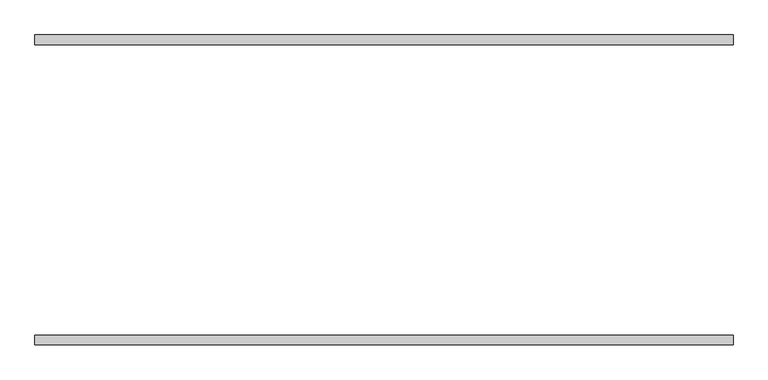
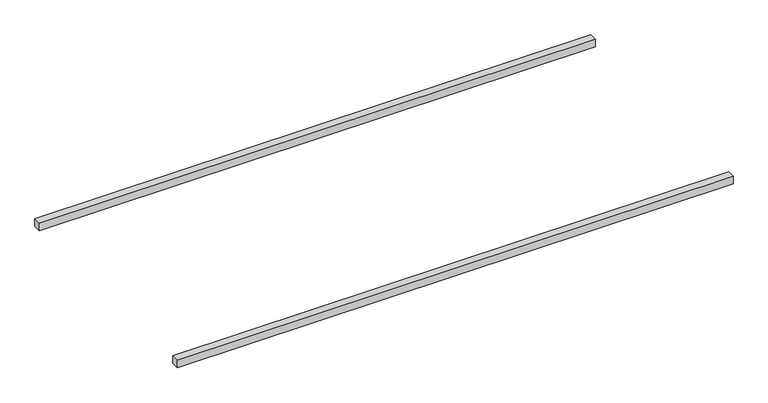
"""IFC4 building model written with IfcOpenShell, lengths in millimetres: furniture geometry."""

from ifc_helpers import new_model, si_unit, frame, origin, place, context, project, spatial, polyline, outline, extrude, source, transform, mapped, element, save


def furniture_1e63cb50(model_context):
    return source(origin(), model_context, "Body", "SweptSolid", [
        extrude(outline(polyline([(583.435329, 475.0), (583.435329, 445.0), (-1556.564671, 445.0), (-1556.564671, 475.0), (583.435329, 475.0)])), frame((0.0, 0.0, 840.0), z_axis=(0.0, 0.0, 1.0), x_axis=(1.0, 0.0, 0.0)), (0.0, 0.0, 1.0), 30.0),
        extrude(outline(polyline([(583.435329, -475.0), (-1556.564671, -475.0), (-1556.564671, -445.0), (583.435329, -445.0), (583.435329, -475.0)])), frame((0.0, 0.0, 840.0), z_axis=(0.0, 0.0, 1.0), x_axis=(1.0, 0.0, 0.0)), (0.0, 0.0, 1.0), 30.0),
    ])


if __name__ == "__main__":
    model = new_model("IFC4")
    model_context = context("Model", 3, world=origin())
    ifc_project = project(units=[si_unit("LENGTHUNIT", "METRE", prefix="MILLI")], contexts=[model_context])
    site = spatial("IfcSite", under=ifc_project)
    building = spatial("IfcBuilding", under=site)
    placement = place(None, origin())
    furniture_shape = furniture_1e63cb50(model_context)
    element("IfcFurniture", 1, at=placement, inside=building, context=model_context, shape_type="MappedRepresentation", body=[
        mapped(furniture_shape, transform((0.0, 0.0, 0.0), x_axis=(1.0, 0.0, 0.0), y_axis=(0.0, 1.0, 0.0), z_axis=(0.0, 0.0, 1.0))),
    ])
    save(model, "model.ifc")

# Revit data of these elements
# Type
#   Stärke Tischplatte = 30 mm
#   Breite von Bein = 30 mm
#   Höhe = 900 mm
#   Länge = 2200 mm
#   Tiefe = 950 mm
#   Seitlicher Versatz Stuhlachse = 400 mm
#   Stühle vorn = yes
#   Stühle seitlich = yes
#   Im Vordergrund zeichnen [instance] = yes
#   Anzahl Stühle pro Seite = 3
#   2 Stühle zentriert = no
#   Tischgestell = none
#   Stuhlbeine = none
#   Default Elevation = 0
#   Assembly Code = ""
